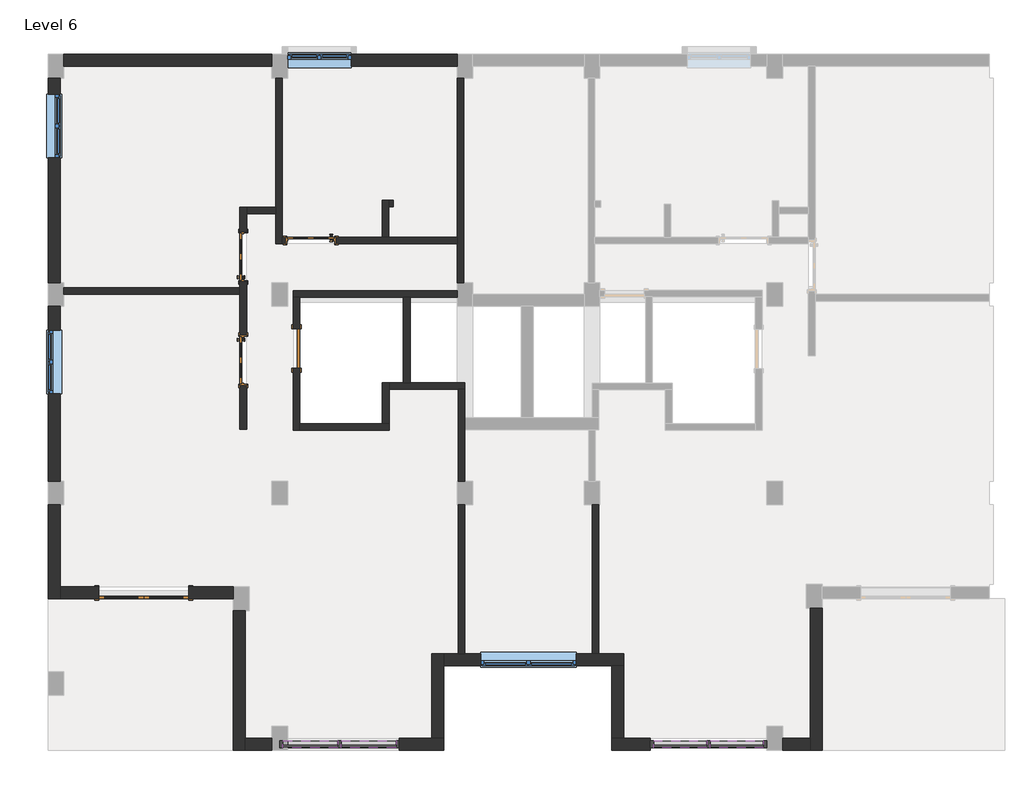
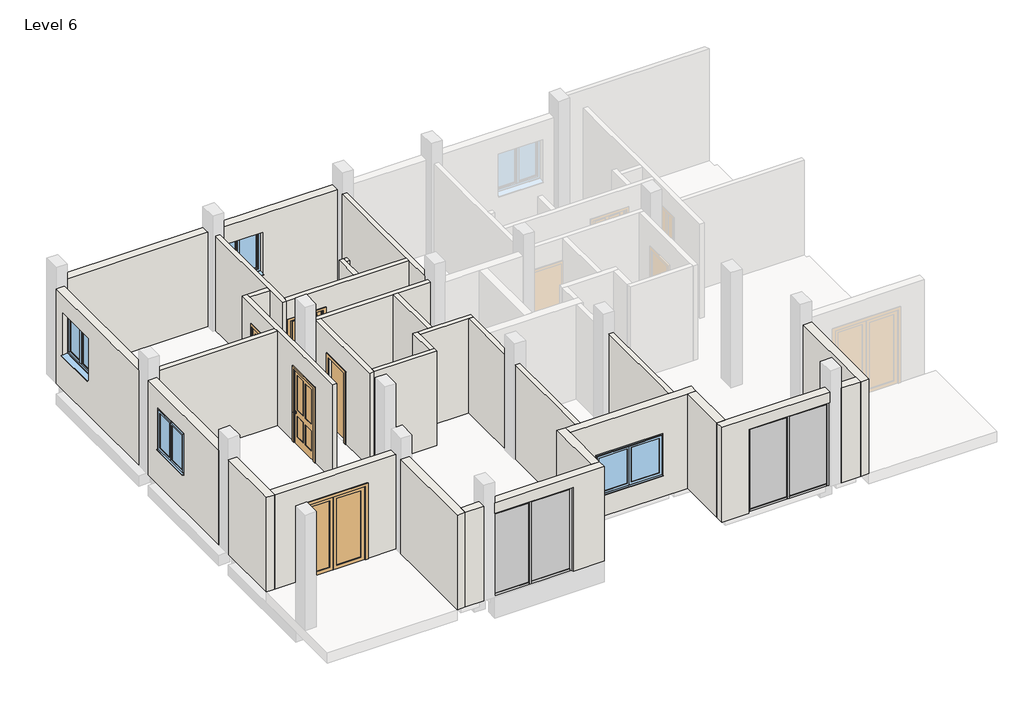
# One storey, part 1 of 3: 32 walls, 14 members, 5 doors, 4 plates, 4 windows.
"""IFC4 building model written with IfcOpenShell, lengths in millimetres."""

from ifc_helpers import new_model, si_unit, frame, origin, place, context, project, spatial, polyline, outline, extrude, faceted_brep, transform, mapped, element, save
from components import door_e52a3823, door_68a706ac, door_a823658d, door_1fe7f57d, member_a1c24a98, member_7fa39cca, member_f0fea5a5, member_ee409385, system_panel_glazed_8311221f, system_panel_glazed_a93c8db9, w2_0001_windows_4_x_4_9dec5fc7, w2_0001_window_4_x_6_83c3b52c

model = new_model("IFC4")

# Units and contexts
model_context = context("Model", 3, world=origin())
ifc_project = project(units=[si_unit("LENGTHUNIT", "METRE", prefix="MILLI")], contexts=[model_context])

# Site, building, storey
site = spatial("IfcSite", under=ifc_project)
building = spatial("IfcBuilding", under=site)
storey = spatial("IfcBuildingStorey", under=building, Name="Level 6", Elevation=9448.8)

# Doors
placement = place(None, origin())
door_shape = door_e52a3823(model_context)
element("IfcDoor", 1, ObjectType="Door-Double-Glass : 68\" x 84\"", at=placement, inside=storey, context=model_context, shape_type="MappedRepresentation", body=[
    mapped(door_shape, transform((-7309.9981098, -11554.5807833, 9448.8), x_axis=(-1.0, 0.0, 0.0), y_axis=(0.0, -1.0, 0.0), z_axis=(0.0, 0.0, 1.0))),
])
door_2_shape = door_68a706ac(model_context)
element("IfcDoor", 2, ObjectType="Door-Interior-Single-4_Panel-Wood : 36\" x 84\"", at=placement, inside=storey, context=model_context, shape_type="MappedRepresentation", body=[
    mapped(door_2_shape, transform((-5402.1925798, -5105.3620333, 9448.8), x_axis=(0.0, 1.0, 0.0), y_axis=(-1.0, 0.0, 0.0), z_axis=(0.0, 0.0, 1.0))),
])
door_3_shape = door_a823658d(model_context)
element("IfcDoor", 3, ObjectType="Door-Interior-Single-4_Panel-Wood : 36\" x 84\"", at=placement, inside=storey, context=model_context, shape_type="MappedRepresentation", body=[
    mapped(door_3_shape, transform((-4103.6175798, -4789.1311634, 9448.8), x_axis=(-1.0, 0.0, 0.0), y_axis=(0.0, -1.0, 0.0), z_axis=(0.0, 0.0, 1.0))),
])
element("IfcDoor", 4, ObjectType="Door-Interior-Single-4_Panel-Wood : 36\" x 84\"", at=placement, inside=storey, context=model_context, shape_type="MappedRepresentation", body=[
    mapped(door_3_shape, transform((-5402.1925798, -7092.9120333, 9448.8), x_axis=(0.0, -1.0, 0.0), y_axis=(1.0, 0.0, 0.0), z_axis=(0.0, 0.0, 1.0))),
])
door_4_shape = door_1fe7f57d(model_context)
element("IfcDoor", 5, ObjectType="Single-Flush : 30\" x 80\"", at=placement, inside=storey, context=model_context, shape_type="MappedRepresentation", body=[
    mapped(door_4_shape, transform((-4379.0950401, -6863.7942903, 9448.8), x_axis=(0.0, -1.0, 0.0), y_axis=(1.0, 0.0, 0.0), z_axis=(0.0, 0.0, 1.0))),
])

# Members
member_shape = member_a1c24a98(model_context)
element("IfcMember", 6, ObjectType="Rectangular Mullion : 2.5\" x 5\" rectangular", at=placement, inside=storey, context=model_context, shape_type="MappedRepresentation", body=[
    mapped(member_shape, transform((2474.9824202, -14462.5402089, 11887.2), x_axis=(0.0, 0.0, 1.0), y_axis=(0.0, 1.0, 0.0), z_axis=(-1.0, 0.0, 0.0))),
])
element("IfcMember", 7, ObjectType="Rectangular Mullion : 2.5\" x 5\" rectangular", at=placement, inside=storey, context=model_context, shape_type="MappedRepresentation", body=[
    mapped(member_shape, transform((3560.8324202, -14462.5402089, 11887.2), x_axis=(0.0, 0.0, 1.0), y_axis=(0.0, 1.0, 0.0), z_axis=(-1.0, 0.0, 0.0))),
])
element("IfcMember", 8, ObjectType="Rectangular Mullion : 2.5\" x 5\" rectangular", at=placement, inside=storey, context=model_context, shape_type="MappedRepresentation", body=[
    mapped(member_shape, transform((4583.1824202, -14462.5402089, 9448.8), x_axis=(0.0, 0.0, -1.0), y_axis=(0.0, 1.0, 0.0), z_axis=(1.0, 0.0, 0.0))),
])
element("IfcMember", 9, ObjectType="Rectangular Mullion : 2.5\" x 5\" rectangular", at=placement, inside=storey, context=model_context, shape_type="MappedRepresentation", body=[
    mapped(member_shape, transform((3497.3324202, -14462.5402089, 9448.8), x_axis=(0.0, 0.0, -1.0), y_axis=(0.0, 1.0, 0.0), z_axis=(1.0, 0.0, 0.0))),
])
member_2_shape = member_7fa39cca(model_context)
element("IfcMember", 10, ObjectType="Rectangular Mullion : 2.5\" x 5\" rectangular", at=placement, inside=storey, context=model_context, shape_type="MappedRepresentation", body=[
    mapped(member_2_shape, transform((-4637.0175798, -14462.5402089, 11887.2), x_axis=(0.0, 0.0, 1.0), y_axis=(0.0, 1.0, 0.0), z_axis=(-1.0, 0.0, 0.0))),
])
element("IfcMember", 11, ObjectType="Rectangular Mullion : 2.5\" x 5\" rectangular", at=placement, inside=storey, context=model_context, shape_type="MappedRepresentation", body=[
    mapped(member_2_shape, transform((-3519.4175798, -14462.5402089, 11887.2), x_axis=(0.0, 0.0, 1.0), y_axis=(0.0, 1.0, 0.0), z_axis=(-1.0, 0.0, 0.0))),
])
element("IfcMember", 12, ObjectType="Rectangular Mullion : 2.5\" x 5\" rectangular", at=placement, inside=storey, context=model_context, shape_type="MappedRepresentation", body=[
    mapped(member_2_shape, transform((-2465.3175798, -14462.5402089, 9448.8), x_axis=(0.0, 0.0, -1.0), y_axis=(0.0, 1.0, 0.0), z_axis=(1.0, 0.0, 0.0))),
])
element("IfcMember", 13, ObjectType="Rectangular Mullion : 2.5\" x 5\" rectangular", at=placement, inside=storey, context=model_context, shape_type="MappedRepresentation", body=[
    mapped(member_2_shape, transform((-3582.9175798, -14462.5402089, 9448.8), x_axis=(0.0, 0.0, -1.0), y_axis=(0.0, 1.0, 0.0), z_axis=(1.0, 0.0, 0.0))),
])
member_3_shape = member_f0fea5a5(model_context)
element("IfcMember", 14, ObjectType="Rectangular Mullion : 2.5\" x 5\" rectangular", at=placement, inside=storey, context=model_context, shape_type="MappedRepresentation", body=[
    mapped(member_3_shape, transform((3529.0824202, -14462.5402089, 9448.8), x_axis=(-1.0, 0.0, 0.0), y_axis=(0.0, 1.0, 0.0), z_axis=(0.0, 0.0, -1.0))),
])
element("IfcMember", 15, ObjectType="Rectangular Mullion : 2.5\" x 5\" rectangular", at=placement, inside=storey, context=model_context, shape_type="MappedRepresentation", body=[
    mapped(member_3_shape, transform((-3551.1675798, -14462.5402089, 9448.8), x_axis=(-1.0, 0.0, 0.0), y_axis=(0.0, 1.0, 0.0), z_axis=(0.0, 0.0, -1.0))),
])
member_4_shape = member_ee409385(model_context)
element("IfcMember", 16, ObjectType="Rectangular Mullion : 2.5\" x 5\" rectangular", at=placement, inside=storey, context=model_context, shape_type="MappedRepresentation", body=[
    mapped(member_4_shape, transform((2411.4824202, -14462.5402089, 9448.8), x_axis=(-1.0, 0.0, 0.0), y_axis=(0.0, 1.0, 0.0), z_axis=(0.0, 0.0, -1.0))),
])
element("IfcMember", 17, ObjectType="Rectangular Mullion : 2.5\" x 5\" rectangular", at=placement, inside=storey, context=model_context, shape_type="MappedRepresentation", body=[
    mapped(member_4_shape, transform((-4700.5175798, -14462.5402089, 9448.8), x_axis=(-1.0, 0.0, 0.0), y_axis=(0.0, 1.0, 0.0), z_axis=(0.0, 0.0, -1.0))),
])
element("IfcMember", 18, ObjectType="Rectangular Mullion : 2.5\" x 5\" rectangular", at=placement, inside=storey, context=model_context, shape_type="MappedRepresentation", body=[
    mapped(member_4_shape, transform((4646.6824202, -14462.5402089, 11887.2), x_axis=(1.0, 0.0, 0.0), y_axis=(0.0, 1.0, 0.0), z_axis=(0.0, 0.0, 1.0))),
])
element("IfcMember", 19, ObjectType="Rectangular Mullion : 2.5\" x 5\" rectangular", at=placement, inside=storey, context=model_context, shape_type="MappedRepresentation", body=[
    mapped(member_4_shape, transform((-2401.8175798, -14462.5402089, 11887.2), x_axis=(1.0, 0.0, 0.0), y_axis=(0.0, 1.0, 0.0), z_axis=(0.0, 0.0, 1.0))),
])

# Plates
system_panel_glazed_shape = system_panel_glazed_8311221f(model_context)
element("IfcPlate", 20, ObjectType="System Panel : Glazed", at=placement, inside=storey, context=model_context, shape_type="MappedRepresentation", body=[
    mapped(system_panel_glazed_shape, transform((4072.0074202, -14462.5402089, 9512.3), x_axis=(-1.0, 0.0, 0.0), y_axis=(0.0, -1.0, 0.0), z_axis=(0.0, 0.0, 1.0))),
])
element("IfcPlate", 21, ObjectType="System Panel : Glazed", at=placement, inside=storey, context=model_context, shape_type="MappedRepresentation", body=[
    mapped(system_panel_glazed_shape, transform((2986.1574202, -14462.5402089, 9512.3), x_axis=(-1.0, 0.0, 0.0), y_axis=(0.0, -1.0, 0.0), z_axis=(0.0, 0.0, 1.0))),
])
system_panel_glazed_2_shape = system_panel_glazed_a93c8db9(model_context)
element("IfcPlate", 22, ObjectType="System Panel : Glazed", at=placement, inside=storey, context=model_context, shape_type="MappedRepresentation", body=[
    mapped(system_panel_glazed_2_shape, transform((-2992.3675798, -14462.5402089, 9512.3), x_axis=(-1.0, 0.0, 0.0), y_axis=(0.0, -1.0, 0.0), z_axis=(0.0, 0.0, 1.0))),
])
element("IfcPlate", 23, ObjectType="System Panel : Glazed", at=placement, inside=storey, context=model_context, shape_type="MappedRepresentation", body=[
    mapped(system_panel_glazed_2_shape, transform((-4109.9675798, -14462.5402089, 9512.3), x_axis=(-1.0, 0.0, 0.0), y_axis=(0.0, -1.0, 0.0), z_axis=(0.0, 0.0, 1.0))),
])

# Walls
element("IfcWall", 24, ObjectType="EXTERIOR WALL 9\"", at=placement, inside=storey, context=model_context, shape_type="SweptSolid", body=[
    extrude(outline(polyline([(-4852.9175798, -1452.2061634), (-8839.9786397, -1452.2061634), (-8839.9786397, -1223.6061634), (-4852.9175798, -1223.6061634), (-4852.9175798, -1452.2061634)])), frame((0.0, 0.0, 9448.8), z_axis=(0.0, 0.0, 1.0), x_axis=(1.0, 0.0, 0.0)), (0.0, 0.0, 1.0), 2743.2),
])
element("IfcWall", 25, ObjectType="EXTERIOR WALL 9\"", at=placement, inside=storey, context=model_context, shape_type="SweptSolid", body=[
    extrude(outline(polyline([(10448.8, -3328.9175798), (10448.8, -4548.1175798), (9448.8, -4548.1175798), (9448.8, -1296.9175798), (12192.0, -1296.9175798), (12192.0, -4548.1175798), (11668.0, -4548.1175798), (11668.0, -3328.9175798), (10448.8, -3328.9175798)])), frame((0.0, -1452.2061634, 0.0), z_axis=(0.0, 1.0, 0.0), x_axis=(0.0, 0.0, 1.0)), (0.0, 0.0, 1.0), 228.6),
])
element("IfcWall", 26, ObjectType="EXTERIOR WALL 9\"", at=placement, inside=storey, context=model_context, shape_type="SweptSolid", body=[
    extrude(outline(polyline([(-1680.8061634, 9448.8), (-5600.6620333, 9448.8), (-5600.6620333, 12192.0), (-1680.8061634, 12192.0), (-1680.8061634, 9448.8)]), holes=[polyline([(-3204.8061634, 10448.8), (-1985.6061634, 10448.8), (-1985.6061634, 11668.0), (-3204.8061634, 11668.0), (-3204.8061634, 10448.8)])]), frame((-9144.7786397, 0.0, 0.0), z_axis=(1.0, 0.0, 0.0), x_axis=(0.0, 1.0, 0.0)), (0.0, 0.0, 1.0), 228.6),
])
element("IfcWall", 27, ObjectType="EXTERIOR WALL 9\"", at=placement, inside=storey, context=model_context, shape_type="SweptSolid", body=[
    extrude(outline(polyline([(-6057.8620333, 9448.8), (-9410.6620333, 9448.8), (-9410.6620333, 12192.0), (-6057.8620333, 12192.0), (-6057.8620333, 9448.8)]), holes=[polyline([(-6515.0620333, 10448.8), (-6515.0620333, 11668.0), (-7734.2620333, 11668.0), (-7734.2620333, 10448.8), (-6515.0620333, 10448.8)])]), frame((-9144.7786397, 0.0, 0.0), z_axis=(1.0, 0.0, 0.0), x_axis=(0.0, 1.0, 0.0)), (0.0, 0.0, 1.0), 228.6),
])
element("IfcWall", 28, ObjectType="EXTERIOR WALL 9\"", at=placement, inside=storey, context=model_context, shape_type="Brep", body=[
    faceted_brep([(-9144.7786397, -9867.8620333, 9448.8), (-9144.7786397, -11671.2620333, 9448.8), (-9144.7786397, -11671.2620333, 12192.0), (-9144.7786397, -9867.8620333, 12192.0), (-8916.1786397, -9867.8620333, 9448.8), (-8916.1786397, -9867.8620333, 12192.0), (-8916.1786397, -11442.6620333, 12192.0), (-8916.1786397, -11671.2620333, 12192.0), (-8916.1786397, -11671.2620333, 9448.8), (-8916.1786397, -11442.6620333, 9448.8)], [[[0, 1, 2, 3]], [[4, 5, 6, 7, 8, 9]], [[1, 0, 4, 9, 8]], [[3, 2, 7, 6, 5]], [[0, 3, 5, 4]], [[2, 1, 8, 7]]]),
])
element("IfcWall", 29, ObjectType="EXTERIOR WALL 9\"", at=placement, inside=storey, context=model_context, shape_type="SweptSolid", body=[
    extrude(outline(polyline([(12192.0, -5589.5175798), (12192.0, -8916.1786397), (9448.8, -8916.1786397), (9448.8, -8173.5981098), (11582.4, -8173.5981098), (11582.4, -6446.3981098), (9448.8, -6446.3981098), (9448.8, -5589.5175798), (12192.0, -5589.5175798)])), frame((0.0, -11671.2620333, 0.0), z_axis=(0.0, 1.0, 0.0), x_axis=(0.0, 0.0, 1.0)), (0.0, 0.0, 1.0), 228.6),
])
element("IfcWall", 30, ObjectType="EXTERIOR WALL 9\"", at=placement, inside=storey, context=model_context, shape_type="Brep", body=[
    faceted_brep([(5484.8824202, -11849.0620333, 9448.8), (5484.8824202, -14348.2402089, 9448.8), (5484.8824202, -14576.8402089, 9448.8), (5484.8824202, -14576.8402089, 12192.0), (5484.8824202, -14348.2402089, 12192.0), (5484.8824202, -11849.0620333, 12192.0), (5713.4824202, -11849.0620333, 9448.8), (5713.4824202, -11849.0620333, 12192.0), (5713.4824202, -14576.8402089, 12192.0), (5713.4824202, -14576.8402089, 9448.8)], [[[0, 1, 2, 3, 4, 5]], [[6, 7, 8, 9]], [[2, 1, 0, 6, 9]], [[5, 4, 3, 8, 7]], [[0, 5, 7, 6]], [[3, 2, 9, 8]]]),
])
element("IfcWall", 31, ObjectType="EXTERIOR WALL 9\"", at=placement, inside=storey, context=model_context, shape_type="SweptSolid", body=[
    extrude(outline(polyline([(5484.8824202, -14576.8402089), (4951.4824202, -14576.8402089), (4951.4824202, -14348.2402089), (5484.8824202, -14348.2402089), (5484.8824202, -14576.8402089)])), frame((0.0, 0.0, 9448.8), z_axis=(0.0, 0.0, 1.0), x_axis=(1.0, 0.0, 0.0)), (0.0, 0.0, 1.0), 2743.2),
])
element("IfcWall", 32, ObjectType="EXTERIOR WALL 9\"", at=placement, inside=storey, context=model_context, shape_type="Brep", body=[
    faceted_brep([(-5589.5175798, -11899.8620333, 9448.8), (-5589.5175798, -14576.8402089, 9448.8), (-5589.5175798, -14576.8402089, 12192.0), (-5589.5175798, -11899.8620333, 12192.0), (-5360.9175798, -11899.8620333, 9448.8), (-5360.9175798, -11899.8620333, 12192.0), (-5360.9175798, -14348.2402089, 12192.0), (-5360.9175798, -14576.8402089, 12192.0), (-5360.9175798, -14576.8402089, 9448.8), (-5360.9175798, -14348.2402089, 9448.8)], [[[0, 1, 2, 3]], [[4, 5, 6, 7, 8, 9]], [[1, 0, 4, 9, 8]], [[3, 2, 7, 6, 5]], [[0, 3, 5, 4]], [[2, 1, 8, 7]]]),
])
element("IfcWall", 33, ObjectType="EXTERIOR WALL 9\"", at=placement, inside=storey, context=model_context, shape_type="SweptSolid", body=[
    extrude(outline(polyline([(-5360.9175798, -14348.2402089), (-4852.9175798, -14348.2402089), (-4852.9175798, -14576.8402089), (-5360.9175798, -14576.8402089), (-5360.9175798, -14348.2402089)])), frame((0.0, 0.0, 9448.8), z_axis=(0.0, 0.0, 1.0), x_axis=(1.0, 0.0, 0.0)), (0.0, 0.0, 1.0), 2743.2),
])
element("IfcWall", 34, ObjectType="EXTERIOR WALL 9\"", at=placement, inside=storey, context=model_context, shape_type="Brep", body=[
    faceted_brep([(1674.8824202, -14348.2402089, 12192.0), (1903.4824202, -14348.2402089, 12192.0), (4646.6824202, -14348.2402089, 12192.0), (4646.6824202, -14348.2402089, 11887.2), (2411.4824202, -14348.2402089, 11887.2), (2411.4824202, -14348.2402089, 9448.8), (1903.4824202, -14348.2402089, 9448.8), (1674.8824202, -14348.2402089, 9448.8), (4646.6824202, -14576.8402089, 12192.0), (1674.8824202, -14576.8402089, 12192.0), (1674.8824202, -14576.8402089, 9448.8), (2411.4824202, -14576.8402089, 9448.8), (2411.4824202, -14576.8402089, 11887.2), (4646.6824202, -14576.8402089, 11887.2)], [[[0, 1, 2, 3, 4, 5, 6, 7]], [[8, 9, 10, 11, 12, 13]], [[10, 7, 6, 5, 11]], [[2, 1, 0, 9, 8]], [[2, 8, 13, 3]], [[0, 7, 10, 9]], [[4, 12, 11, 5]], [[12, 4, 3, 13]]]),
])
element("IfcWall", 35, ObjectType="EXTERIOR WALL 9\"", at=placement, inside=storey, context=model_context, shape_type="Brep", body=[
    faceted_brep([(-1550.9175798, -14576.8402089, 12192.0), (-4548.1175798, -14576.8402089, 12192.0), (-4548.1175798, -14576.8402089, 11887.2), (-2401.8175798, -14576.8402089, 11887.2), (-2401.8175798, -14576.8402089, 9448.8), (-1550.9175798, -14576.8402089, 9448.8), (-4548.1175798, -14348.2402089, 12192.0), (-1779.5175798, -14348.2402089, 12192.0), (-1550.9175798, -14348.2402089, 12192.0), (-1550.9175798, -14348.2402089, 9448.8), (-1779.5175798, -14348.2402089, 9448.8), (-2401.8175798, -14348.2402089, 9448.8), (-2401.8175798, -14348.2402089, 11887.2), (-4548.1175798, -14348.2402089, 11887.2)], [[[0, 1, 2, 3, 4, 5]], [[6, 7, 8, 9, 10, 11, 12, 13]], [[9, 5, 4, 11, 10]], [[1, 0, 8, 7, 6]], [[1, 6, 13, 2]], [[0, 5, 9, 8]], [[3, 12, 11, 4]], [[12, 3, 2, 13]]]),
])
element("IfcWall", 36, ObjectType="EXTERIOR WALL 9\"", at=placement, inside=storey, context=model_context, shape_type="Brep", body=[
    faceted_brep([(-1550.9175798, -14348.2402089, 9448.8), (-1550.9175798, -12951.2402089, 9448.8), (-1550.9175798, -12722.6402089, 9448.8), (-1550.9175798, -12722.6402089, 12192.0), (-1550.9175798, -12951.2402089, 12192.0), (-1550.9175798, -14348.2402089, 12192.0), (-1779.5175798, -14348.2402089, 9448.8), (-1779.5175798, -14348.2402089, 12192.0), (-1779.5175798, -12722.6402089, 12192.0), (-1779.5175798, -12722.6402089, 9448.8)], [[[0, 1, 2, 3, 4, 5]], [[6, 7, 8, 9]], [[2, 1, 0, 6, 9]], [[5, 4, 3, 8, 7]], [[0, 5, 7, 6]], [[3, 2, 9, 8]]]),
])
element("IfcWall", 37, ObjectType="EXTERIOR WALL 9\"", at=placement, inside=storey, context=model_context, shape_type="Brep", body=[
    faceted_brep([(-1550.9175798, -12951.2402089, 9448.8), (1674.8824202, -12951.2402089, 9448.8), (1903.4824202, -12951.2402089, 9448.8), (1903.4824202, -12951.2402089, 12192.0), (1674.8824202, -12951.2402089, 12192.0), (-1550.9175798, -12951.2402089, 12192.0), (-839.7175798, -12951.2402089, 10058.4), (-839.7175798, -12951.2402089, 11277.6), (989.0824202, -12951.2402089, 11277.6), (989.0824202, -12951.2402089, 10058.4), (-1550.9175798, -12722.6402089, 9448.8), (-1550.9175798, -12722.6402089, 12192.0), (-1271.5175798, -12722.6402089, 12192.0), (-1144.5175798, -12722.6402089, 12192.0), (1293.8824202, -12722.6402089, 12192.0), (1420.8824202, -12722.6402089, 12192.0), (1903.4824202, -12722.6402089, 12192.0), (1903.4824202, -12722.6402089, 9448.8), (1420.8824202, -12722.6402089, 9448.8), (1293.8824202, -12722.6402089, 9448.8), (-1144.5175798, -12722.6402089, 9448.8), (-1271.5175798, -12722.6402089, 9448.8), (-839.7175798, -12722.6402089, 10058.4), (989.0824202, -12722.6402089, 10058.4), (989.0824202, -12722.6402089, 11277.6), (-839.7175798, -12722.6402089, 11277.6)], [[[0, 1, 2, 3, 4, 5], [6, 7, 8, 9]], [[10, 11, 12, 13, 14, 15, 16, 17, 18, 19, 20, 21], [22, 23, 24, 25]], [[2, 1, 0, 10, 21, 20, 19, 18, 17]], [[5, 4, 3, 16, 15, 14, 13, 12, 11]], [[0, 5, 11, 10]], [[3, 2, 17, 16]], [[7, 6, 22, 25]], [[8, 7, 25, 24]], [[9, 8, 24, 23]], [[6, 9, 23, 22]]]),
])
element("IfcWall", 38, ObjectType="EXTERIOR WALL 9\"", at=placement, inside=storey, context=model_context, shape_type="SweptSolid", body=[
    extrude(outline(polyline([(1674.8824202, -14348.2402089), (1674.8824202, -12951.2402089), (1903.4824202, -12951.2402089), (1903.4824202, -14348.2402089), (1674.8824202, -14348.2402089)])), frame((0.0, 0.0, 9448.8), z_axis=(0.0, 0.0, 1.0), x_axis=(1.0, 0.0, 0.0)), (0.0, 0.0, 1.0), 2743.2),
])
element("IfcWall", 39, ObjectType="INTERIOR WALL 5\"", at=placement, inside=storey, context=model_context, shape_type="SweptSolid", body=[
    extrude(outline(polyline([(-5462.5175798, -5829.2620333), (-8839.9786397, -5829.2620333), (-8839.9786397, -5702.2620333), (-5462.5175798, -5702.2620333), (-5462.5175798, -5829.2620333)])), frame((0.0, 0.0, 9448.8), z_axis=(0.0, 0.0, 1.0), x_axis=(1.0, 0.0, 0.0)), (0.0, 0.0, 1.0), 2743.2),
])
element("IfcWall", 40, ObjectType="INTERIOR WALL 5\"", at=placement, inside=storey, context=model_context, shape_type="Brep", body=[
    faceted_brep([(-5462.5175798, -8420.0620333, 9448.8), (-5462.5175798, -8420.0620333, 12192.0), (-5462.5175798, -5829.2620333, 12192.0), (-5462.5175798, -5702.2620333, 12192.0), (-5462.5175798, -4153.3104011, 12192.0), (-5462.5175798, -4153.3104011, 9448.8), (-5462.5175798, -4622.7620333, 9448.8), (-5462.5175798, -4622.7620333, 11607.8), (-5462.5175798, -5587.9620333, 11607.8), (-5462.5175798, -5587.9620333, 9448.8), (-5462.5175798, -5702.2620333, 9448.8), (-5462.5175798, -5829.2620333, 9448.8), (-5462.5175798, -6610.3120333, 9448.8), (-5462.5175798, -6610.3120333, 11607.8), (-5462.5175798, -7575.5120333, 11607.8), (-5462.5175798, -7575.5120333, 9448.8), (-5335.5175798, -8420.0620333, 12192.0), (-5335.5175798, -8420.0620333, 9448.8), (-5335.5175798, -7575.5120333, 9448.8), (-5335.5175798, -7575.5120333, 11607.8), (-5335.5175798, -6610.3120333, 11607.8), (-5335.5175798, -6610.3120333, 9448.8), (-5335.5175798, -5587.9620333, 9448.8), (-5335.5175798, -5587.9620333, 11607.8), (-5335.5175798, -4622.7620333, 11607.8), (-5335.5175798, -4622.7620333, 9448.8), (-5335.5175798, -4280.3104011, 9448.8), (-5335.5175798, -4153.3104011, 9448.8), (-5335.5175798, -4153.3104011, 12192.0), (-5335.5175798, -4280.3104011, 12192.0)], [[[0, 1, 2, 3, 4, 5, 6, 7, 8, 9, 10, 11, 12, 13, 14, 15]], [[16, 17, 18, 19, 20, 21, 22, 23, 24, 25, 26, 27, 28, 29]], [[17, 0, 15, 18]], [[5, 27, 26, 25, 6]], [[9, 22, 21, 12, 11, 10]], [[1, 0, 17, 16]], [[4, 3, 2, 1, 16, 29, 28]], [[5, 4, 28, 27]], [[24, 7, 6, 25]], [[7, 24, 23, 8]], [[8, 23, 22, 9]], [[14, 19, 18, 15]], [[19, 14, 13, 20]], [[20, 13, 12, 21]]]),
])
element("IfcWall", 41, ObjectType="INTERIOR WALL 5\"", at=placement, inside=storey, context=model_context, shape_type="SweptSolid", body=[
    extrude(outline(polyline([(-4776.7175798, -4280.3104011), (-5335.5175798, -4280.3104011), (-5335.5175798, -4153.3104011), (-4776.7175798, -4153.3104011), (-4776.7175798, -4280.3104011)])), frame((0.0, 0.0, 9448.8), z_axis=(0.0, 0.0, 1.0), x_axis=(1.0, 0.0, 0.0)), (0.0, 0.0, 1.0), 2743.2),
])
element("IfcWall", 42, ObjectType="INTERIOR WALL 5\"", at=placement, inside=storey, context=model_context, shape_type="Brep", body=[
    faceted_brep([(-4776.7175798, -1680.8061634, 9448.8), (-4776.7175798, -4153.3104011, 9448.8), (-4776.7175798, -4280.3104011, 9448.8), (-4776.7175798, -4855.8061634, 9448.8), (-4776.7175798, -4855.8061634, 12192.0), (-4776.7175798, -4280.3104011, 12192.0), (-4776.7175798, -4153.3104011, 12192.0), (-4776.7175798, -1680.8061634, 12192.0), (-4649.7175798, -1680.8061634, 9448.8), (-4649.7175798, -1680.8061634, 12192.0), (-4649.7175798, -4728.8061634, 12192.0), (-4649.7175798, -4855.8061634, 12192.0), (-4649.7175798, -4855.8061634, 9448.8), (-4649.7175798, -4728.8061634, 9448.8)], [[[0, 1, 2, 3, 4, 5, 6, 7]], [[8, 9, 10, 11, 12, 13]], [[3, 2, 1, 0, 8, 13, 12]], [[7, 6, 5, 4, 11, 10, 9]], [[0, 7, 9, 8]], [[4, 3, 12, 11]]]),
])
element("IfcWall", 43, ObjectType="INTERIOR WALL 5\"", at=placement, inside=storey, context=model_context, shape_type="Brep", body=[
    faceted_brep([(-1296.9175798, -4855.8061634, 12192.0), (-4649.7175798, -4855.8061634, 12192.0), (-4649.7175798, -4855.8061634, 9448.8), (-4586.2175798, -4855.8061634, 9448.8), (-4586.2175798, -4855.8061634, 11607.8), (-3621.0175798, -4855.8061634, 11607.8), (-3621.0175798, -4855.8061634, 9448.8), (-1296.9175798, -4855.8061634, 9448.8), (-4649.7175798, -4728.8061634, 12192.0), (-2732.0175798, -4728.8061634, 12192.0), (-2605.0175798, -4728.8061634, 12192.0), (-1296.9175798, -4728.8061634, 12192.0), (-1296.9175798, -4728.8061634, 9448.8), (-2605.0175798, -4728.8061634, 9448.8), (-2732.0175798, -4728.8061634, 9448.8), (-3621.0175798, -4728.8061634, 9448.8), (-3621.0175798, -4728.8061634, 11607.8), (-4586.2175798, -4728.8061634, 11607.8), (-4586.2175798, -4728.8061634, 9448.8), (-4649.7175798, -4728.8061634, 9448.8)], [[[0, 1, 2, 3, 4, 5, 6, 7]], [[8, 9, 10, 11, 12, 13, 14, 15, 16, 17, 18, 19]], [[2, 19, 18, 3]], [[12, 7, 6, 15, 14, 13]], [[1, 0, 11, 10, 9, 8]], [[2, 1, 8, 19]], [[0, 7, 12, 11]], [[17, 4, 3, 18]], [[4, 17, 16, 5]], [[5, 16, 15, 6]]]),
])
element("IfcWall", 44, ObjectType="INTERIOR WALL 5\"", at=placement, inside=storey, context=model_context, shape_type="Brep", body=[
    faceted_brep([(-1296.9175798, -1680.8061634, 9448.8), (-1296.9175798, -4728.8061634, 9448.8), (-1296.9175798, -4855.8061634, 9448.8), (-1296.9175798, -5600.6620333, 9448.8), (-1296.9175798, -5600.6620333, 12192.0), (-1296.9175798, -4855.8061634, 12192.0), (-1296.9175798, -4728.8061634, 12192.0), (-1296.9175798, -1680.8061634, 12192.0), (-1169.9175798, -1680.8061634, 9448.8), (-1169.9175798, -1680.8061634, 12192.0), (-1169.9175798, -5600.6620333, 12192.0), (-1169.9175798, -5600.6620333, 9448.8)], [[[0, 1, 2, 3, 4, 5, 6, 7]], [[8, 9, 10, 11]], [[3, 2, 1, 0, 8, 11]], [[4, 3, 11, 10]], [[7, 6, 5, 4, 10, 9]], [[0, 7, 9, 8]]]),
])
element("IfcWall", 45, ObjectType="INTERIOR WALL 5\"", at=placement, inside=storey, context=model_context, shape_type="Brep", body=[
    faceted_brep([(-2605.0175798, -4728.8061634, 9448.8), (-2605.0175798, -4144.6061634, 9448.8), (-2605.0175798, -4017.6061634, 9448.8), (-2605.0175798, -4017.6061634, 12192.0), (-2605.0175798, -4144.6061634, 12192.0), (-2605.0175798, -4728.8061634, 12192.0), (-2732.0175798, -4728.8061634, 9448.8), (-2732.0175798, -4728.8061634, 12192.0), (-2732.0175798, -4017.6061634, 12192.0), (-2732.0175798, -4017.6061634, 9448.8)], [[[0, 1, 2, 3, 4, 5]], [[6, 7, 8, 9]], [[2, 1, 0, 6, 9]], [[5, 4, 3, 8, 7]], [[0, 5, 7, 6]], [[3, 2, 9, 8]]]),
])
element("IfcWall", 46, ObjectType="INTERIOR WALL 5\"", at=placement, inside=storey, context=model_context, shape_type="SweptSolid", body=[
    extrude(outline(polyline([(-2605.0175798, -4017.6061634), (-2516.1175798, -4017.6061634), (-2516.1175798, -4144.6061634), (-2605.0175798, -4144.6061634), (-2605.0175798, -4017.6061634)])), frame((0.0, 0.0, 9448.8), z_axis=(0.0, 0.0, 1.0), x_axis=(1.0, 0.0, 0.0)), (0.0, 0.0, 1.0), 2743.2),
])
element("IfcWall", 47, ObjectType="INTERIOR WALL 5\"", at=placement, inside=storey, context=model_context, shape_type="Brep", body=[
    faceted_brep([(-4442.5950401, -5885.8942903, 9448.8), (-4315.5950401, -5885.8942903, 9448.8), (-2325.6175798, -5885.8942903, 9448.8), (-2198.6175798, -5885.8942903, 9448.8), (-1296.9175798, -5885.8942903, 9448.8), (-1296.9175798, -5885.8942903, 12192.0), (-2198.6175798, -5885.8942903, 12192.0), (-2325.6175798, -5885.8942903, 12192.0), (-4315.5950401, -5885.8942903, 12192.0), (-4442.5950401, -5885.8942903, 12192.0), (-4442.5950401, -5758.8942903, 9448.8), (-4442.5950401, -5758.8942903, 12192.0), (-1296.9175798, -5758.8942903, 12192.0), (-1296.9175798, -5758.8942903, 9448.8)], [[[0, 1, 2, 3, 4, 5, 6, 7, 8, 9]], [[10, 11, 12, 13]], [[4, 3, 2, 1, 0, 10, 13]], [[5, 4, 13, 12]], [[9, 8, 7, 6, 5, 12, 11]], [[0, 9, 11, 10]]]),
])
element("IfcWall", 48, ObjectType="INTERIOR WALL 5\"", at=placement, inside=storey, context=model_context, shape_type="Brep", body=[
    faceted_brep([(-4442.5950401, -7244.7942903, 11480.8), (-4442.5950401, -7244.7942903, 9448.8), (-4442.5950401, -8439.1120333, 9448.8), (-4442.5950401, -8439.1120333, 12192.0), (-4442.5950401, -5885.8942903, 12192.0), (-4442.5950401, -5885.8942903, 9448.8), (-4442.5950401, -6482.7942903, 9448.8), (-4442.5950401, -6482.7942903, 11480.8), (-4315.5950401, -8439.1120333, 9448.8), (-4315.5950401, -8312.1120333, 9448.8), (-4315.5950401, -7244.7942903, 9448.8), (-4315.5950401, -7244.7942903, 11480.8), (-4315.5950401, -6482.7942903, 11480.8), (-4315.5950401, -6482.7942903, 9448.8), (-4315.5950401, -5885.8942903, 9448.8), (-4315.5950401, -5885.8942903, 12192.0), (-4315.5950401, -8312.1120333, 12192.0), (-4315.5950401, -8439.1120333, 12192.0)], [[[0, 1, 2, 3, 4, 5, 6, 7]], [[8, 9, 10, 11, 12, 13, 14, 15, 16, 17]], [[6, 5, 14, 13]], [[2, 1, 10, 9, 8]], [[4, 3, 17, 16, 15]], [[5, 4, 15, 14]], [[3, 2, 8, 17]], [[11, 10, 1, 0]], [[12, 11, 0, 7]], [[13, 12, 7, 6]]]),
])
element("IfcWall", 49, ObjectType="INTERIOR WALL 5\"", at=placement, inside=storey, context=model_context, shape_type="Brep", body=[
    faceted_brep([(-4315.5950401, -8439.1120333, 9448.8), (-2601.0950401, -8439.1120333, 9448.8), (-2601.0950401, -8439.1120333, 12192.0), (-4315.5950401, -8439.1120333, 12192.0), (-4315.5950401, -8312.1120333, 9448.8), (-4315.5950401, -8312.1120333, 12192.0), (-2728.0950401, -8312.1120333, 12192.0), (-2601.0950401, -8312.1120333, 12192.0), (-2601.0950401, -8312.1120333, 9448.8), (-2728.0950401, -8312.1120333, 9448.8)], [[[0, 1, 2, 3]], [[4, 5, 6, 7, 8, 9]], [[1, 0, 4, 9, 8]], [[3, 2, 7, 6, 5]], [[0, 3, 5, 4]], [[2, 1, 8, 7]]]),
])
element("IfcWall", 50, ObjectType="INTERIOR WALL 5\"", at=placement, inside=storey, context=model_context, shape_type="Brep", body=[
    faceted_brep([(-2601.0950401, -8312.1120333, 9448.8), (-2601.0950401, -7651.7120333, 9448.8), (-2601.0950401, -7524.7120333, 9448.8), (-2601.0950401, -7524.7120333, 12192.0), (-2601.0950401, -7651.7120333, 12192.0), (-2601.0950401, -8312.1120333, 12192.0), (-2728.0950401, -8312.1120333, 9448.8), (-2728.0950401, -8312.1120333, 12192.0), (-2728.0950401, -7524.7120333, 12192.0), (-2728.0950401, -7524.7120333, 9448.8)], [[[0, 1, 2, 3, 4, 5]], [[6, 7, 8, 9]], [[2, 1, 0, 6, 9]], [[5, 4, 3, 8, 7]], [[0, 5, 7, 6]], [[3, 2, 9, 8]]]),
])
element("IfcWall", 51, ObjectType="INTERIOR WALL 5\"", at=placement, inside=storey, context=model_context, shape_type="Brep", body=[
    faceted_brep([(-2601.0950401, -7651.7120333, 9448.8), (-1271.5175798, -7651.7120333, 9448.8), (-1144.5175798, -7651.7120333, 9448.8), (-1144.5175798, -7651.7120333, 12192.0), (-1271.5175798, -7651.7120333, 12192.0), (-2601.0950401, -7651.7120333, 12192.0), (-2601.0950401, -7524.7120333, 9448.8), (-2601.0950401, -7524.7120333, 12192.0), (-2325.6175798, -7524.7120333, 12192.0), (-2198.6175798, -7524.7120333, 12192.0), (-1144.5175798, -7524.7120333, 12192.0), (-1144.5175798, -7524.7120333, 9448.8), (-2198.6175798, -7524.7120333, 9448.8), (-2325.6175798, -7524.7120333, 9448.8)], [[[0, 1, 2, 3, 4, 5]], [[6, 7, 8, 9, 10, 11, 12, 13]], [[2, 1, 0, 6, 13, 12, 11]], [[5, 4, 3, 10, 9, 8, 7]], [[0, 5, 7, 6]], [[3, 2, 11, 10]]]),
])
element("IfcWall", 52, ObjectType="INTERIOR WALL 5\"", at=placement, inside=storey, context=model_context, shape_type="SweptSolid", body=[
    extrude(outline(polyline([(-2325.6175798, -7524.7120333), (-2325.6175798, -5885.8942903), (-2198.6175798, -5885.8942903), (-2198.6175798, -7524.7120333), (-2325.6175798, -7524.7120333)])), frame((0.0, 0.0, 9448.8), z_axis=(0.0, 0.0, 1.0), x_axis=(1.0, 0.0, 0.0)), (0.0, 0.0, 1.0), 2743.2),
])
element("IfcWall", 53, ObjectType="INTERIOR WALL 5\"", at=placement, inside=storey, context=model_context, shape_type="Brep", body=[
    faceted_brep([(-1271.5175798, -7651.7120333, 9448.8), (-1271.5175798, -9417.0120333, 9448.8), (-1271.5175798, -9417.0120333, 12192.0), (-1271.5175798, -7651.7120333, 12192.0), (-1144.5175798, -7651.7120333, 9448.8), (-1144.5175798, -7651.7120333, 12192.0), (-1144.5175798, -8197.8120333, 12192.0), (-1144.5175798, -8426.4120333, 12192.0), (-1144.5175798, -9417.0120333, 12192.0), (-1144.5175798, -9417.0120333, 9448.8), (-1144.5175798, -8426.4120333, 9448.8), (-1144.5175798, -8197.8120333, 9448.8)], [[[0, 1, 2, 3]], [[4, 5, 6, 7, 8, 9, 10, 11]], [[1, 0, 4, 11, 10, 9]], [[2, 1, 9, 8]], [[3, 2, 8, 7, 6, 5]], [[0, 3, 5, 4]]]),
])
element("IfcWall", 54, ObjectType="INTERIOR WALL 5\"", at=placement, inside=storey, context=model_context, shape_type="SweptSolid", body=[
    extrude(outline(polyline([(-1271.5175798, -12722.6402089), (-1271.5175798, -9867.8620333), (-1144.5175798, -9867.8620333), (-1144.5175798, -12722.6402089), (-1271.5175798, -12722.6402089)])), frame((0.0, 0.0, 9448.8), z_axis=(0.0, 0.0, 1.0), x_axis=(1.0, 0.0, 0.0)), (0.0, 0.0, 1.0), 2743.2),
])
element("IfcWall", 55, ObjectType="INTERIOR WALL 5\"", at=placement, inside=storey, context=model_context, shape_type="SweptSolid", body=[
    extrude(outline(polyline([(1293.8824202, -12722.6402089), (1293.8824202, -9867.8620333), (1420.8824202, -9867.8620333), (1420.8824202, -12722.6402089), (1293.8824202, -12722.6402089)])), frame((0.0, 0.0, 9448.8), z_axis=(0.0, 0.0, 1.0), x_axis=(1.0, 0.0, 0.0)), (0.0, 0.0, 1.0), 2743.2),
])

# Windows
w2_0001_windows_4_x_4_shape = w2_0001_windows_4_x_4_9dec5fc7(model_context)
element("IfcWindow", 56, ObjectType="w2.0001 : WINDOWS 4' X 4'", at=placement, inside=storey, context=model_context, shape_type="MappedRepresentation", body=[
    mapped(w2_0001_windows_4_x_4_shape, transform((-9030.4786397, -2595.2061634, 9448.8), x_axis=(0.0, 1.0, 0.0), y_axis=(-1.0, 0.0, 0.0), z_axis=(0.0, 0.0, 1.0))),
])
element("IfcWindow", 57, ObjectType="w2.0001 : WINDOWS 4' X 4'", at=placement, inside=storey, context=model_context, shape_type="MappedRepresentation", body=[
    mapped(w2_0001_windows_4_x_4_shape, transform((-9030.4786397, -7124.6620333, 9448.8), x_axis=(0.0, -1.0, 0.0), y_axis=(1.0, 0.0, 0.0), z_axis=(0.0, 0.0, 1.0))),
])
element("IfcWindow", 58, ObjectType="w2.0001 : WINDOWS 4' X 4'", at=placement, inside=storey, context=model_context, shape_type="MappedRepresentation", body=[
    mapped(w2_0001_windows_4_x_4_shape, transform((-3938.5175798, -1337.9061634, 9448.8), x_axis=(-1.0, 0.0, 0.0), y_axis=(0.0, -1.0, 0.0), z_axis=(0.0, 0.0, 1.0))),
])
w2_0001_window_4_x_6_shape = w2_0001_window_4_x_6_83c3b52c(model_context)
element("IfcWindow", 59, ObjectType="w2.0001 : window 4' x 6'", at=placement, inside=storey, context=model_context, shape_type="MappedRepresentation", body=[
    mapped(w2_0001_window_4_x_6_shape, transform((74.6824202, -12836.9402089, 9058.4), x_axis=(1.0, 0.0, 0.0), y_axis=(0.0, 1.0, 0.0), z_axis=(0.0, 0.0, 1.0))),
])

save(model, "model.ifc")

# Revit data of these elements
# Type "Door-Double-Glass : 68\" x 84\""
#   Type Mark = "11"
#   Construction Type Id = "opn-d45"
#   Assembly Code = "C1020"
#   Analytic Construction = "Wood frame, double glass door "
#   W = 2' - 10"
#   Thickness = 0' - 2"
#   Thermal Resistance (R) = 1.8150 (h·ft²·°F)/BTU
#   Swing Angle [instance default] = 90.00°
#   Heat Transfer Coefficient (U) = 0.5510 BTU/(h·ft²·°F)
#   Height = 7' - 0"
#   Bottom Rail = 0' - 4"
#   Top Rail = 0' - 4"
#   Stiles = 0' - 4"
#   Trim Projection = 0' - 1"
#   Trim Width = 0' - 3"
#   Width = 5' - 8"
#   Define Thermal Properties by = 1
#   Glazing = Glass
#   Panel Material = Wood - Birch - Solid Stained Light Low Gloss
#   Trim Material = Paint - Sienna
#   Visual Light Transmittance = 0
#   Solar Heat Gain Coefficient = 0
#   Function = (empty or 0)
#   Wall Closure = (empty or 0)
# Type "Door-Interior-Single-4_Panel-Wood : 36\" x 84\""
#   Type Mark = "9"
#   Assembly Code = "C1020300"
#   Analytic Construction = "Wooden"
#   Top Rail = 0' - 4 11/16"
#   Thickness = 0' - 1 3/8"
#   Thermal Resistance (R) = 2.5876 (h·ft²·°F)/BTU
#   Swing Angle [instance default] = 90.00°
#   Stiles = 0' - 4 3/4"
#   Rough Width = 3' - 2"
#   Rough Height = 7' - 1"
#   Mullion = 0' - 4 1/2"
#   Lock Rail = 0' - 7 1/2"
#   Height = 7' - 0"
#   Width = 3' - 0"
#   Heat Transfer Coefficient (U) = 0.3865 BTU/(h·ft²·°F)
#   Bottom Rail = 0' - 9 1/8"
#   Trim Material = Cherry
#   Panel Material = Cherry
#   Frame Material = Cherry
#   Door Handle Material = Aluminum
#   Visual Light Transmittance = 0
#   Solar Heat Gain Coefficient = 0
#   Wall Closure = (empty or 0)
#   Function = (empty or 0)
# Type "Single-Flush : 30\" x 80\""
#   Type Mark = "5"
#   Construction Type Id = "MDOOR"
#   Assembly Code = "C1020"
#   Analytic Construction = "Metal"
#   Thickness = 0' - 2"
#   Heat Transfer Coefficient (U) = 0.651978 BTU/(h·ft²·°F)
#   Height = 6' - 8"
#   Trim Projection Ext = 0' - 1"
#   Trim Projection Int = 0' - 1"
#   Trim Width = 0' - 3"
#   Width = 2' - 6"
#   Define Thermal Properties by = 1
#   Define Thermal Properties by = 1
#   Door Material = Door - Panel
#   Frame Material = Door - Frame
#   Visual Light Transmittance = 0
#   Solar Heat Gain Coefficient = 0
#   Function = (empty or 0)
#   Wall Closure = (empty or 0)
# Type "Rectangular Mullion : 2.5\" x 5\" rectangular"
#   built-in parameter 1007304 = 0.416667 (stored number, unit not read)
#   built-in parameter 1007301 = 0.104167 (stored number, unit not read)
#   built-in parameter 1007300 = 0.104167 (stored number, unit not read)
# Type "System Panel : Glazed"
#   Construction Type Id = "GSP4R"
#   Analytic Construction = "1/8 in Pilkington single glazing"
#   Visual Light Transmittance = 0.9
#   Solar Heat Gain Coefficient = 0.86
#   Heat Transfer Coefficient (U) = 1.18115 BTU/(h·ft²·°F)
#   Define Thermal Properties by = 1
# Type "EXTERIOR WALL 9\""
#   Assembly Code = "B2010"
#   Layers, outside or top first: 0' - 9" "WARM BEIGE COLOUR" (function 1)
# Type "INTERIOR WALL 5\""
#   Assembly Code = "B2010"
#   Layers, outside or top first: 0' - 5" "WARM BEIGE COLOUR" (function 1)
# Type "w2.0001 : WINDOWS 4' X 4'"
#   Type Mark = "21"
#   Operation = "DoublePanelVertical"
#   Keynote = "16.05.01"
#   Analytic Construction = "<None>"
#   Rough Width = 4' - 0"
#   Rough Height = 4' - 0"
#   Rahmentiefe = 0' - 2.3622"
#   Rahmenhöhe unten = 0' - 3.14961"
#   Rahmehöhe oben = 0' - 3.14961"
#   Rahmenbreite = 0' - 2.3622"
#   Height = 4' - 0"
#   Flügeltiefe = 0' - 2.3622"
#   Flügelbreite = 0' - 2.3622"
#   Einbautiefe (von außen) [instance default] = 0' - 5.51181"
#   Width = 4' - 0"
#   Kippflügel [instance default] = yes
#   Drehflügel im Grundriß darstellen [instance default] = no
#   Drehflügel [instance default] = yes
#   Define Thermal Properties by = 1
#   Rahmen [instance default] = none
#   Glas [instance default] = none
#   Flügel [instance default] = none
#   Fensterbank aussen [instance default] = none
#   Fensterbank innen [instance default] = none
#   Wall Closure = (empty or 0)
# Type "w2.0001 : window 4' x 6'"
#   Type Mark = "22"
#   Operation = "DoublePanelVertical"
#   Keynote = "16.05.01"
#   Analytic Construction = "<None>"
#   Rough Width = 6' - 0"
#   Rough Height = 4' - 0"
#   Rahmentiefe = 0' - 2.3622"
#   Rahmenhöhe unten = 0' - 3.14961"
#   Rahmehöhe oben = 0' - 3.14961"
#   Rahmenbreite = 0' - 2.3622"
#   Height = 4' - 0"
#   Flügeltiefe = 0' - 2.3622"
#   Flügelbreite = 0' - 2.3622"
#   Einbautiefe (von außen) [instance default] = 0' - 5.51181"
#   Width = 6' - 0"
#   Kippflügel [instance default] = yes
#   Drehflügel im Grundriß darstellen [instance default] = no
#   Drehflügel [instance default] = yes
#   Define Thermal Properties by = 1
#   Rahmen [instance default] = none
#   Glas [instance default] = none
#   Flügel [instance default] = none
#   Fensterbank aussen [instance default] = none
#   Fensterbank innen [instance default] = none
#   Wall Closure = (empty or 0)
# Element 1 (IfcDoor, "Door-Double-Glass : 68\" x 84\"")
#   Phase Created = New Construction
#   Materials on its faces: "Wood - Birch - Solid Stained Light Low Gloss", "Paint - Sienna", "Glass"
# Elements 2, 3, 4 (IfcDoor, "Door-Interior-Single-4_Panel-Wood : 36\" x 84\"")
#   Swing Angle = 90.00°
#   Phase Created = New Construction
#   Materials on its faces: "Cherry", "Aluminum"
# Element 5 (IfcDoor, "Single-Flush : 30\" x 80\"")
#   Phase Created = New Construction
#   Materials on its faces: "Door - Frame", "Door - Panel"
# Elements 6, 7, 8, 9, 10, 11, 12, 13, 14, 15, 16, 17, 18, 19 (IfcMember, "Rectangular Mullion : 2.5\" x 5\" rectangular")
#   Phase Created = New Construction
#   Materials on its faces: "Aluminum"
# Elements 20, 21, 22, 23 (IfcPlate, "System Panel : Glazed")
#   Phase Created = New Construction
#   Materials on its faces: "Glass"
# Elements 24, 25, 26, 27, 28, 29, 30, 31, 32, 33, 34, 35, 36, 37, 38 (IfcWall, "EXTERIOR WALL 9\"")
#   Top Offset = 9' - 0"
#   Base Offset = 0' - 0"
#   wall height = 9' - 0"
#   Phase Created = New Construction
#   Base Constraint = Level 6
#   Top Constraint = Level 6
#   Materials on its faces: "WARM BEIGE COLOUR"
# Elements 39, 40, 41, 42, 43, 44, 45, 46, 47, 48, 49, 50, 51, 52, 53, 54, 55 (IfcWall, "INTERIOR WALL 5\"")
#   Top Offset = 9' - 0"
#   Base Offset = 0' - 0"
#   wall height = 9' - 0"
#   Phase Created = New Construction
#   Base Constraint = Level 6
#   Top Constraint = Level 6
#   Materials on its faces: "WARM BEIGE COLOUR"
# Element 56 (IfcWindow, "w2.0001 : WINDOWS 4' X 4'")
#   Mark = "33"
#   Einbautiefe (von außen) = 0' - 5.51181"
#   Kippflügel = yes
#   Drehflügel im Grundriß darstellen = no
#   Drehflügel = yes
#   Rahmen = none
#   Glas = none
#   Flügel = none
#   Fensterbank innen = none
#   Fensterbank aussen = none
#   Phase Created = New Construction
#   Materials on its faces: "Fenster - Kunststoff", "Fenster - Kunststoff weiss", "Glass", "Fenster - Holz"
# Element 57 (IfcWindow, "w2.0001 : WINDOWS 4' X 4'")
#   Mark = "34"
#   Einbautiefe (von außen) = 0' - 5.51181"
#   Kippflügel = yes
#   Drehflügel im Grundriß darstellen = no
#   Drehflügel = yes
#   Rahmen = none
#   Glas = none
#   Flügel = none
#   Fensterbank innen = none
#   Fensterbank aussen = none
#   Phase Created = New Construction
#   Materials on its faces: "Fenster - Kunststoff", "Fenster - Kunststoff weiss", "Glass", "Fenster - Holz"
# Element 58 (IfcWindow, "w2.0001 : WINDOWS 4' X 4'")
#   Mark = "38"
#   Einbautiefe (von außen) = 0' - 5.51181"
#   Kippflügel = yes
#   Drehflügel im Grundriß darstellen = no
#   Drehflügel = yes
#   Rahmen = none
#   Glas = none
#   Flügel = none
#   Fensterbank innen = none
#   Fensterbank aussen = none
#   Phase Created = New Construction
#   Materials on its faces: "Fenster - Kunststoff", "Fenster - Kunststoff weiss", "Glass", "Fenster - Holz"
# Element 59 (IfcWindow, "w2.0001 : window 4' x 6'")
#   Mark = "43"
#   Einbautiefe (von außen) = 0' - 5.51181"
#   Kippflügel = yes
#   Drehflügel im Grundriß darstellen = no
#   Drehflügel = yes
#   Rahmen = none
#   Glas = none
#   Flügel = none
#   Fensterbank innen = none
#   Fensterbank aussen = none
#   Phase Created = New Construction
#   Materials on its faces: "Fenster - Kunststoff", "Fenster - Kunststoff weiss", "Glass", "Fenster - Holz"
# Materials
#   "Glass": class "Glass", colour RGB 0 128 192, transparency 0.75, Description = "Soda Lime Glass", Cost = 0
#   "Wood - Birch - Solid Stained Light Low Gloss": class "Wood", colour RGB 210 159 95, transparency 0, Cost = 0
#   "Paint - Sienna": colour RGB 118 70 51, transparency 0, Cost = 0
#   "Cherry": class "Wood", colour RGB 226 177 128, transparency 0, Description = "Prunus Serotina", Cost = 0
#   "Aluminum": class "Metal", colour RGB 247 247 247, transparency 0, Description = "Aluminum 6061", Cost = 0
#   "Door - Panel": class "Wood", colour RGB 210 159 95, transparency 0, Cost = 0
#   "Door - Frame": colour RGB 118 70 51, transparency 0, Cost = 0
#   "WARM BEIGE COLOUR": class "Generic", colour RGB 120 120 120, transparency 0, Cost = 0
#   "Fenster - Kunststoff": colour RGB 249 249 249, transparency 0
#   "Fenster - Kunststoff weiss": colour RGB 249 249 249, transparency 0
#   "Fenster - Holz": colour RGB 216 135 75, transparency 0
